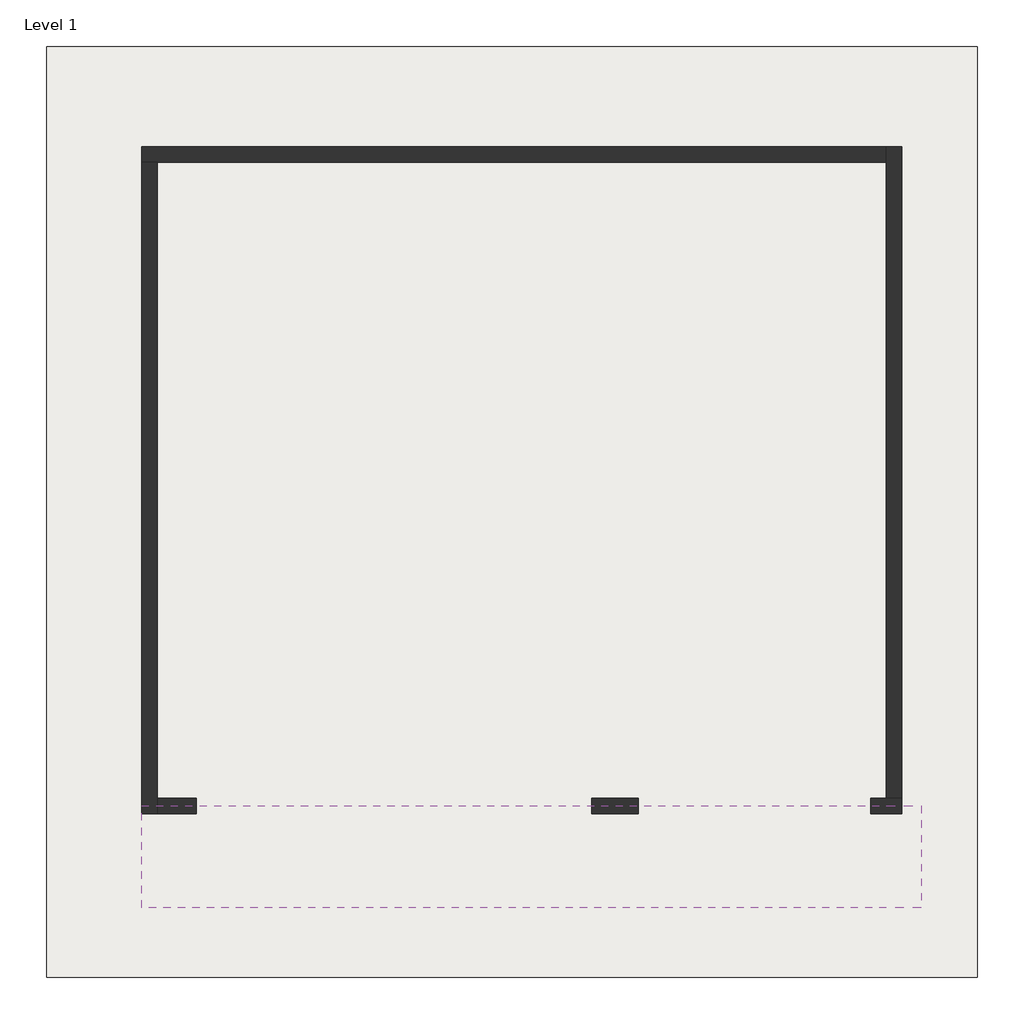
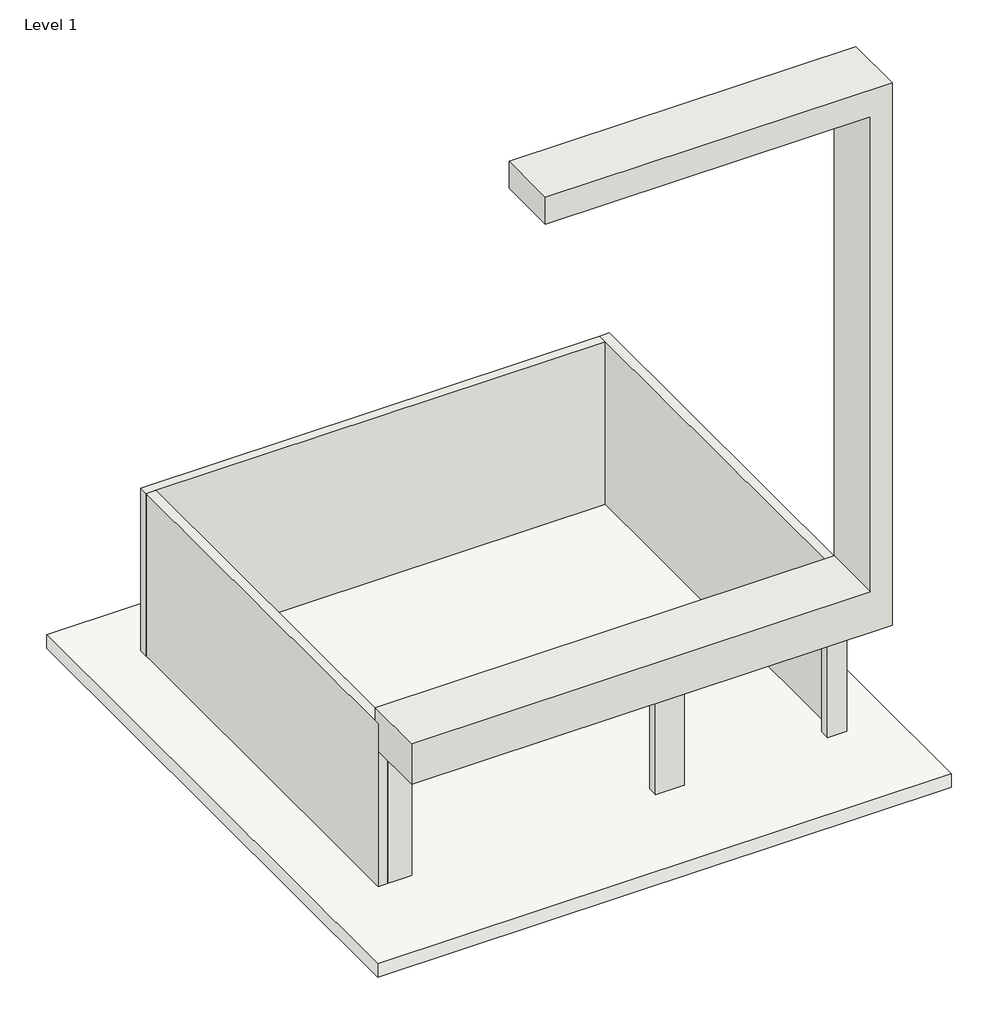
# One storey: 5 walls, 1 slab.
"""IFC4 building model written with IfcOpenShell, lengths in millimetres."""

from ifc_helpers import new_model, si_unit, frame, origin, place, context, project, spatial, polyline, outline, extrude, faceted_brep, transform, mapped, element, save
from components import walls_2_walls_2_e5515708

model = new_model("IFC4")

# Units and contexts
model_context = context("Model", 3, world=origin())
ifc_project = project(units=[si_unit("LENGTHUNIT", "METRE", prefix="MILLI")], contexts=[model_context])

# Site, building, storey
site = spatial("IfcSite", under=ifc_project)
building = spatial("IfcBuilding", under=site)
storey = spatial("IfcBuildingStorey", under=building, Name="Level 1", Elevation=0.0)

# Slab
placement = place(None, origin())
element("IfcSlab", 1, ObjectType="Generic - 12\"", at=placement, inside=storey, context=model_context, shape_type="SweptSolid", body=[
    extrude(outline(polyline([(-1353.9492777, 11320.6421898), (-1353.9492777, -871.3578102), (-13545.9492777, -871.3578102), (-13545.9492777, 11320.6421898), (-1353.9492777, 11320.6421898)])), frame((0.0, 0.0, -304.8), z_axis=(0.0, 0.0, 1.0), x_axis=(1.0, 0.0, 0.0)), (0.0, 0.0, 1.0), 304.8),
])

# Walls
element("IfcWall", 2, ObjectType="Generic - 8\"", at=placement, inside=storey, context=model_context, shape_type="Brep", body=[
    faceted_brep([(-12299.7432037, 9807.0548743, 0.0), (-12096.5432037, 9807.0548743, 0.0), (-2546.1432037, 9807.0548743, 0.0), (-2546.1432037, 9807.0548743, 3657.6), (-12096.5432037, 9807.0548743, 3657.6), (-12299.7432037, 9807.0548743, 3657.6), (-12299.7432037, 10010.2548743, 0.0), (-12299.7432037, 10010.2548743, 3657.6), (-2546.1432037, 10010.2548743, 3657.6), (-2546.1432037, 10010.2548743, 0.0)], [[[0, 1, 2, 3, 4, 5]], [[6, 7, 8, 9]], [[2, 1, 0, 6, 9]], [[0, 5, 7, 6]], [[3, 2, 9, 8]], [[5, 4, 3, 8, 7]]]),
])
element("IfcWall", 3, ObjectType="Generic - 8\"", at=placement, inside=storey, context=model_context, shape_type="Brep", body=[
    faceted_brep([(-12096.5432037, 1272.6548743, 0.0), (-12096.5432037, 1475.8548743, 0.0), (-12096.5432037, 9807.0548743, 0.0), (-12096.5432037, 9807.0548743, 3657.6), (-12096.5432037, 1475.8548743, 3657.6), (-12096.5432037, 1272.6548743, 3657.6), (-12299.7432037, 1272.6548743, 0.0), (-12299.7432037, 1272.6548743, 3657.6), (-12299.7432037, 9807.0548743, 3657.6), (-12299.7432037, 9807.0548743, 0.0)], [[[0, 1, 2, 3, 4, 5]], [[6, 7, 8, 9]], [[2, 1, 0, 6, 9]], [[0, 5, 7, 6]], [[3, 2, 9, 8]], [[5, 4, 3, 8, 7]]]),
])
element("IfcWall", 4, ObjectType="Generic - 8\"", at=placement, inside=storey, context=model_context, shape_type="Brep", body=[
    faceted_brep([(-2342.9432037, 1475.8548743, 0.0), (-2546.1432037, 1475.8548743, 0.0), (-2749.3432037, 1475.8548743, 0.0), (-2749.3432037, 1475.8548743, 3048.0), (-5797.3432037, 1475.8548743, 3048.0), (-5797.3432037, 1475.8548743, 0.0), (-6406.9432037, 1475.8548743, 0.0), (-6406.9432037, 1475.8548743, 3048.0), (-11588.5432037, 1475.8548743, 3048.0), (-11588.5432037, 1475.8548743, 0.0), (-12096.5432037, 1475.8548743, 0.0), (-12096.5432037, 1475.8548743, 3657.6), (-2546.1432037, 1475.8548743, 3657.6), (-2342.9432037, 1475.8548743, 3657.6), (-2342.9432037, 1272.6548743, 0.0), (-2342.9432037, 1272.6548743, 3657.6), (-12096.5432037, 1272.6548743, 3657.6), (-12096.5432037, 1272.6548743, 0.0), (-11588.5432037, 1272.6548743, 0.0), (-11588.5432037, 1272.6548743, 3048.0), (-6406.9432037, 1272.6548743, 3048.0), (-6406.9432037, 1272.6548743, 0.0), (-5797.3432037, 1272.6548743, 0.0), (-5797.3432037, 1272.6548743, 3048.0), (-2749.3432037, 1272.6548743, 3048.0), (-2749.3432037, 1272.6548743, 0.0)], [[[0, 1, 2, 3, 4, 5, 6, 7, 8, 9, 10, 11, 12, 13]], [[14, 15, 16, 17, 18, 19, 20, 21, 22, 23, 24, 25]], [[0, 13, 15, 14]], [[11, 10, 17, 16]], [[13, 12, 11, 16, 15]], [[2, 1, 0, 14, 25]], [[3, 2, 25, 24]], [[4, 3, 24, 23]], [[5, 4, 23, 22]], [[6, 5, 22, 21]], [[7, 6, 21, 20]], [[8, 7, 20, 19]], [[9, 8, 19, 18]], [[10, 9, 18, 17]]]),
])
element("IfcWall", 5, ObjectType="Generic - 8\"", at=placement, inside=storey, context=model_context, shape_type="Brep", body=[
    faceted_brep([(-2546.1432037, 10010.2548743, 0.0), (-2546.1432037, 9807.0548743, 0.0), (-2546.1432037, 1475.8548743, 0.0), (-2546.1432037, 1475.8548743, 3657.6), (-2546.1432037, 9807.0548743, 3657.6), (-2546.1432037, 10010.2548743, 3657.6), (-2342.9432037, 10010.2548743, 0.0), (-2342.9432037, 10010.2548743, 3657.6), (-2342.9432037, 1475.8548743, 3657.6), (-2342.9432037, 1475.8548743, 0.0)], [[[0, 1, 2, 3, 4, 5]], [[6, 7, 8, 9]], [[2, 1, 0, 6, 9]], [[0, 5, 7, 6]], [[3, 2, 9, 8]], [[5, 4, 3, 8, 7]]]),
])
walls_2_walls_2_shape = walls_2_walls_2_e5515708(model_context)
element("IfcWall", 6, ObjectType="Walls 2 : Walls 2", at=placement, inside=storey, context=model_context, shape_type="MappedRepresentation", body=[
    mapped(walls_2_walls_2_shape, transform((0.0, 0.0, 0.0), x_axis=(1.0, 0.0, 0.0), y_axis=(0.0, 1.0, 0.0), z_axis=(0.0, 0.0, 1.0))),
])

save(model, "model.ifc")

# Revit data of these elements
# Type "Generic - 12\""
#   Assembly Code = "B1010"
#   Function = 0
#   Layers, outside or top first: 1' - 0" no material (function 1)
# Type "Generic - 8\""
#   Assembly Code = "B2010"
#   Layers, outside or top first: 0' - 8" no material (function 1)
# Element 1 (IfcSlab, "Generic - 12\"")
#   Height Offset From Level = 0' - 0"
#   Phase Created = New Construction
#   Materials on its faces: "Default Floor"
# Elements 2, 3, 4, 5 (IfcWall, "Generic - 8\"")
#   Top Offset = 0' - 0"
#   Base Offset = 0' - 0"
#   Unconnected Height = 12' - 0"
#   wall height = 12' - 0"
#   Phase Created = New Construction
#   Base Constraint = Level 1
#   Materials on its faces: "Default Wall"
# Element 6 (IfcWall, "Walls 2 : Walls 2")
#   Phase Created = New Construction
#   Materials on its faces: "Default Wall"
# Materials
#   "Default Floor": colour RGB 128 128 128, transparency 0
#   "Default Wall": colour RGB 128 128 128, transparency 0
